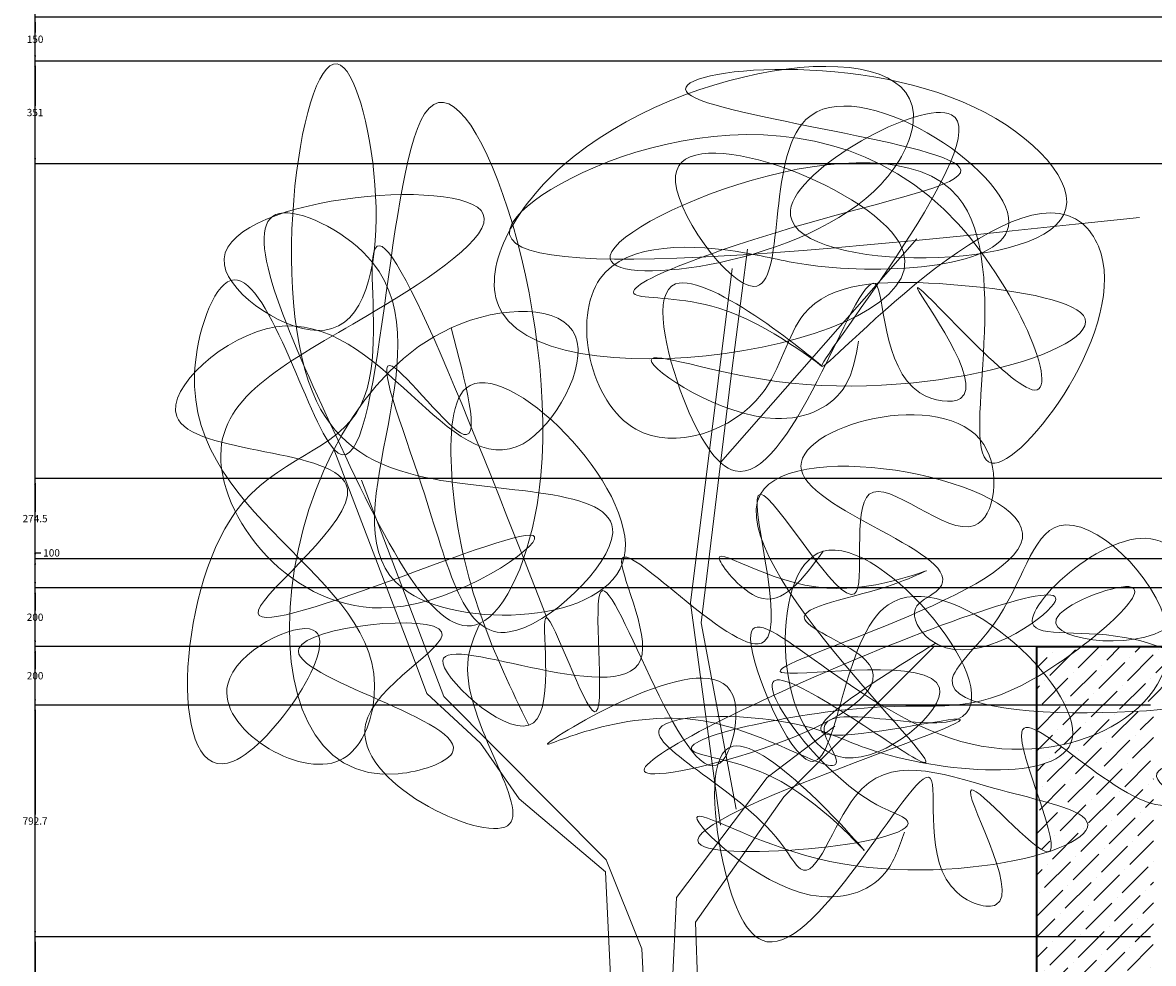
# Model space of a CAD drawing. Units: millimetres. Extents: x -692 to 9639, y -141 to 10345.
# Tile 2 of 19: x -692 to 3174, y 1765 to 4981. Entities that reach past the tile are written whole.
import ezdxf

# ---------------------------------------------------------------- set-up
doc = ezdxf.new("R2010")
doc.units = ezdxf.units.MM
doc.header["$MEASUREMENT"] = 0
for name, color, linetype, lineweight in [('A-ANNO-DIMS', 2, 'Continuous', 18), ('A-ELEV', 7, 'Continuous', 35), ('A-ELEV-PATT', 8, 'Continuous', 13), ('L-PLNT', 3, 'Continuous', 18)]:
    doc.layers.add(name, color=color, linetype=linetype, lineweight=lineweight)
doc.styles.get("Standard").update_dxf_attribs({"font": 'arial.ttf'})
doc.dimstyles.get("Standard").update_dxf_attribs({"dimtxt": 25, "dimasz": 20, "dimexe": 0.18, "dimexo": 10, "dimgap": 10, "dimtad": 0, "dimtih": 1, "dimtoh": 1, "dimdec": 0, "dimzin": 0, "dimdsep": 46, "dimtxsty": 'Standard', "dimcen": 10, "dimadec": 0, "dimazin": 0, "dimtfac": 1, "dimtdec": 0, "dimtofl": 0, "dimtmove": 0, "dimatfit": 3, "dimfxl": 1, "dimtolj": 1, "dimtzin": 0, "dimarcsym": 0})

# ---------------------------------------------------------------- blocks, each defined once
blk = doc.blocks.new('*D7')
at = {"layer": 'A-ANNO-DIMS', "color": 0, "lineweight": -2, "transparency": 16777216}
for p, q in [((8481.5, 9848.8), (-649.1, 9848.8)), ((-648.9, 9828.8), (-648.9, 5124.9)), ((-648.9, 375.6), (-648.9, 5079.4)), ((2463.7, 355.6), (-649.1, 355.6))]:
    blk.add_line(p, q, dxfattribs=at)
at = {"layer": 'A-ANNO-DIMS', "color": 0, "lineweight": -3, "transparency": 16777216}
for points in [[(-652.2, 9828.8), (-645.6, 9828.8), (-648.9, 9848.8)], [(-652.2, 375.6), (-645.6, 375.6), (-648.9, 355.6)]]:
    blk.add_solid(points, dxfattribs=at)
at = {"layer": 'Defpoints', "color": 0, "lineweight": -3, "transparency": 16777216}
for p in [(-648.9, 9848.8), (8491.5, 9848.8), (2473.7, 355.6)]:
    blk.add_point(p, dxfattribs=at)
at = {"layer": 'A-ANNO-DIMS', "color": 0, "transparency": 16777216, "insert": (-648.9, 5102.2), "char_height": 25, "attachment_point": 5}
blk.add_mtext('\\A1;9493', dxfattribs=at)
blk = doc.blocks.new('*D25')
at = {"layer": 'A-ANNO-DIMS', "color": 0, "lineweight": -2, "transparency": 16777216}
for p, q in [((3163.7, 1855.6), (-649.1, 1855.6)), ((-648.9, 1835.6), (-648.9, 1378.3)), ((-648.9, 875.6), (-648.9, 1332.8)), ((2763.7, 855.6), (-649.1, 855.6))]:
    blk.add_line(p, q, dxfattribs=at)
at = {"layer": 'A-ANNO-DIMS', "color": 0, "lineweight": -3, "transparency": 16777216}
for points in [[(-652.2, 1835.6), (-645.6, 1835.6), (-648.9, 1855.6)], [(-652.2, 875.6), (-645.6, 875.6), (-648.9, 855.6)]]:
    blk.add_solid(points, dxfattribs=at)
at = {"layer": 'Defpoints', "color": 0, "lineweight": -3, "transparency": 16777216}
for p in [(-648.9, 1855.6), (3173.7, 1855.6), (2773.7, 855.6)]:
    blk.add_point(p, dxfattribs=at)
at = {"layer": 'A-ANNO-DIMS', "color": 0, "transparency": 16777216, "insert": (-648.9, 1355.6), "char_height": 25, "attachment_point": 5}
blk.add_mtext('\\A1;1000', dxfattribs=at)
blk = doc.blocks.new('*D26')
at = {"layer": 'A-ANNO-DIMS', "color": 0, "lineweight": -2, "transparency": 16777216}
for p, q in [((3163.7, 2648.3), (-649.1, 2648.3)), ((-648.9, 2628.3), (-648.9, 2274.7)), ((-648.9, 1875.6), (-648.9, 2229.2)), ((3163.7, 1855.6), (-649.1, 1855.6))]:
    blk.add_line(p, q, dxfattribs=at)
at = {"layer": 'A-ANNO-DIMS', "color": 0, "lineweight": -3, "transparency": 16777216}
for points in [[(-652.2, 2628.3), (-645.6, 2628.3), (-648.9, 2648.3)], [(-652.2, 1875.6), (-645.6, 1875.6), (-648.9, 1855.6)]]:
    blk.add_solid(points, dxfattribs=at)
at = {"layer": 'Defpoints', "color": 0, "lineweight": -3, "transparency": 16777216}
for p in [(-648.9, 2648.3), (3173.7, 2648.3), (3173.7, 1855.6)]:
    blk.add_point(p, dxfattribs=at)
at = {"layer": 'A-ANNO-DIMS', "color": 0, "transparency": 16777216, "insert": (-648.9, 2251.9), "char_height": 25, "attachment_point": 5}
blk.add_mtext('\\A1;792.7', dxfattribs=at)
blk = doc.blocks.new('*D27')
at = {"layer": 'A-ANNO-DIMS', "color": 0, "lineweight": -2, "transparency": 16777216}
for p, q in [((2763.7, 2848.3), (-649.1, 2848.3)), ((-648.9, 2828.3), (-648.9, 2771)), ((-648.9, 2668.3), (-648.9, 2725.5)), ((3163.7, 2648.3), (-649.1, 2648.3))]:
    blk.add_line(p, q, dxfattribs=at)
at = {"layer": 'A-ANNO-DIMS', "color": 0, "lineweight": -3, "transparency": 16777216}
for points in [[(-652.2, 2828.3), (-645.6, 2828.3), (-648.9, 2848.3)], [(-652.2, 2668.3), (-645.6, 2668.3), (-648.9, 2648.3)]]:
    blk.add_solid(points, dxfattribs=at)
at = {"layer": 'Defpoints', "color": 0, "lineweight": -3, "transparency": 16777216}
for p in [(-648.9, 2848.3), (2773.7, 2848.3), (3173.7, 2648.3)]:
    blk.add_point(p, dxfattribs=at)
at = {"layer": 'A-ANNO-DIMS', "color": 0, "transparency": 16777216, "insert": (-648.9, 2748.3), "char_height": 25, "attachment_point": 5}
blk.add_mtext('\\A1;200', dxfattribs=at)
blk = doc.blocks.new('*D59')
at = {"layer": 'A-ANNO-DIMS', "color": 0, "lineweight": -2, "transparency": 16777216}
for p, q in [((5031.5, 3048.3), (-649.1, 3048.3)), ((-648.9, 3028.3), (-648.9, 2971)), ((-648.9, 2868.3), (-648.9, 2925.5)), ((3181.5, 2848.3), (-649.1, 2848.3))]:
    blk.add_line(p, q, dxfattribs=at)
at = {"layer": 'A-ANNO-DIMS', "color": 0, "lineweight": -3, "transparency": 16777216}
for points in [[(-652.2, 3028.3), (-645.6, 3028.3), (-648.9, 3048.3)], [(-652.2, 2868.3), (-645.6, 2868.3), (-648.9, 2848.3)]]:
    blk.add_solid(points, dxfattribs=at)
at = {"layer": 'Defpoints', "color": 0, "lineweight": -3, "transparency": 16777216}
for p in [(-648.9, 3048.3), (5041.5, 3048.3), (3191.5, 2848.3)]:
    blk.add_point(p, dxfattribs=at)
at = {"layer": 'A-ANNO-DIMS', "color": 0, "transparency": 16777216, "insert": (-648.9, 2948.3), "char_height": 25, "attachment_point": 5}
blk.add_mtext('\\A1;200', dxfattribs=at)
blk = doc.blocks.new('*D60')
at = {"layer": 'A-ANNO-DIMS', "color": 0, "lineweight": -2, "transparency": 16777216}
for p, q in [((5031.5, 3148.3), (-649.1, 3148.3)), ((-648.9, 3148.3), (-648.9, 3168.3)), ((-648.9, 3168.3), (-628.9, 3168.3)), ((-648.9, 3068.3), (-648.9, 3128.3)), ((5031.5, 3048.3), (-649.1, 3048.3))]:
    blk.add_line(p, q, dxfattribs=at)
at = {"layer": 'A-ANNO-DIMS', "color": 0, "lineweight": -3, "transparency": 16777216}
for points in [[(-652.2, 3128.3), (-645.6, 3128.3), (-648.9, 3148.3)], [(-652.2, 3068.3), (-645.6, 3068.3), (-648.9, 3048.3)]]:
    blk.add_solid(points, dxfattribs=at)
at = {"layer": 'Defpoints', "color": 0, "lineweight": -3, "transparency": 16777216}
for p in [(-648.9, 3148.3), (5041.5, 3148.3), (5041.5, 3048.3)]:
    blk.add_point(p, dxfattribs=at)
at = {"layer": 'A-ANNO-DIMS', "color": 0, "transparency": 16777216, "insert": (-592.5, 3168.3), "char_height": 25, "attachment_point": 5}
blk.add_mtext('\\A1;100', dxfattribs=at)
blk = doc.blocks.new('*D61')
at = {"layer": 'A-ANNO-DIMS', "color": 0, "lineweight": -2, "transparency": 16777216}
for p, q in [((3931.5, 3422.8), (-649.1, 3422.8)), ((-648.9, 3402.8), (-648.9, 3308.3)), ((-648.9, 3168.3), (-648.9, 3262.8)), ((5031.5, 3148.3), (-649.1, 3148.3))]:
    blk.add_line(p, q, dxfattribs=at)
at = {"layer": 'A-ANNO-DIMS', "color": 0, "lineweight": -3, "transparency": 16777216}
for points in [[(-652.2, 3402.8), (-645.6, 3402.8), (-648.9, 3422.8)], [(-652.2, 3168.3), (-645.6, 3168.3), (-648.9, 3148.3)]]:
    blk.add_solid(points, dxfattribs=at)
at = {"layer": 'Defpoints', "color": 0, "lineweight": -3, "transparency": 16777216}
for p in [(-648.9, 3422.8), (3941.5, 3422.8), (5041.5, 3148.3)]:
    blk.add_point(p, dxfattribs=at)
at = {"layer": 'A-ANNO-DIMS', "color": 0, "transparency": 16777216, "insert": (-648.9, 3285.5), "char_height": 25, "attachment_point": 5}
blk.add_mtext('\\A1;274.5', dxfattribs=at)
blk = doc.blocks.new('*D62')
at = {"layer": 'A-ANNO-DIMS', "color": 0, "lineweight": -2, "transparency": 16777216}
for p, q in [((3781.5, 4848.8), (-649.1, 4848.8)), ((-648.9, 4828.8), (-648.9, 4696)), ((-648.9, 4517.8), (-648.9, 4650.5)), ((3931.5, 4497.8), (-649.1, 4497.8))]:
    blk.add_line(p, q, dxfattribs=at)
at = {"layer": 'A-ANNO-DIMS', "color": 0, "lineweight": -3, "transparency": 16777216}
for points in [[(-652.2, 4828.8), (-645.6, 4828.8), (-648.9, 4848.8)], [(-652.2, 4517.8), (-645.6, 4517.8), (-648.9, 4497.8)]]:
    blk.add_solid(points, dxfattribs=at)
at = {"layer": 'Defpoints', "color": 0, "lineweight": -3, "transparency": 16777216}
for p in [(-648.9, 4848.8), (3791.5, 4848.8), (3941.5, 4497.8)]:
    blk.add_point(p, dxfattribs=at)
at = {"layer": 'A-ANNO-DIMS', "color": 0, "transparency": 16777216, "insert": (-648.9, 4673.3), "char_height": 25, "attachment_point": 5}
blk.add_mtext('\\A1;351', dxfattribs=at)
blk = doc.blocks.new('*D63')
at = {"layer": 'A-ANNO-DIMS', "color": 0, "lineweight": -2, "transparency": 16777216}
for p, q in [((3931.5, 4998.8), (-649.1, 4998.8)), ((-648.9, 4978.8), (-648.9, 4946.5)), ((-648.9, 4868.8), (-648.9, 4901)), ((3781.5, 4848.8), (-649.1, 4848.8))]:
    blk.add_line(p, q, dxfattribs=at)
at = {"layer": 'A-ANNO-DIMS', "color": 0, "lineweight": -3, "transparency": 16777216}
for points in [[(-652.2, 4978.8), (-645.6, 4978.8), (-648.9, 4998.8)], [(-652.2, 4868.8), (-645.6, 4868.8), (-648.9, 4848.8)]]:
    blk.add_solid(points, dxfattribs=at)
at = {"layer": 'Defpoints', "color": 0, "lineweight": -3, "transparency": 16777216}
for p in [(-648.9, 4998.8), (3941.5, 4998.8), (3791.5, 4848.8)]:
    blk.add_point(p, dxfattribs=at)
at = {"layer": 'A-ANNO-DIMS', "color": 0, "transparency": 16777216, "insert": (-648.9, 4923.8), "char_height": 25, "attachment_point": 5}
blk.add_mtext('\\A1;150', dxfattribs=at)

msp = doc.modelspace()

# ---------------------------------------------------------------- hatches: boundary and pattern name
at = {"layer": 'A-ELEV-PATT'}
h = msp.add_hatch(dxfattribs=at)
h.set_pattern_fill('ANSI36', color=256, scale=400)
edge = h.paths.add_edge_path()
edge.add_spline(control_points=[(3173.746, 2309.965), (3085.901, 2332.226), (2969.139, 2424.713), (2876.436, 2493.45)], knot_values=[20955.88576955, 20955.88576955, 20955.88576955, 20955.88576955, 21219.85539585, 21219.85539585, 21219.85539585, 21219.85539585], degree=3, periodic=0)
edge.add_spline(control_points=[(2876.436, 2493.45), (2855.134, 2468.311), (2819.135, 2451.154), (2773.746, 2440.514)], knot_values=[5238.08213467, 5238.08213467, 5238.08213467, 5238.08213467, 5382.8513026, 5382.8513026, 5382.8513026, 5382.8513026], degree=3, periodic=0)
edge.add_line((2773.746, 2440.514), (2773.746, 2354.397))
edge.add_spline(control_points=[(2773.746, 2354.397), (2777.278, 2343.918), (2780.812, 2333.449), (2784.279, 2323.093)], knot_values=[20514.20511429, 20514.20511429, 20514.20511429, 20514.20511429, 20537.39604293, 20537.39604293, 20537.39604293, 20537.39604293], degree=3, periodic=0)
edge.add_spline(control_points=[(2784.279, 2323.093), (2849.257, 2305.468), (3007.384, 2255.171), (2928.441, 2185.016), (2819.76, 2148.371)], knot_values=[1896.27813718, 1896.27813718, 1896.27813718, 1896.27813718, 2077.70067144, 2424.51760392, 2424.51760392, 2424.51760392, 2424.51760392], degree=3, periodic=0)
edge.add_spline(control_points=[(2819.76, 2148.371), (2817.899, 2146.748), (2815.52, 2145.926), (2812.57, 2145.987)], knot_values=[20304.87329269, 20304.87329269, 20304.87329269, 20304.87329269, 20326.21847821, 20326.21847821, 20326.21847821, 20326.21847821], degree=3, periodic=0)
edge.add_spline(control_points=[(2812.57, 2145.987), (2800.291, 2141.985), (2787.329, 2138.102), (2773.746, 2134.363)], knot_values=[1850.39591646, 1850.39591646, 1850.39591646, 1850.39591646, 1888.716341, 1888.716341, 1888.716341, 1888.716341], degree=3, periodic=0)
edge.add_line((2773.746, 2134.363), (2773.746, 855.575))
edge.add_line((2773.746, 855.575), (3173.746, 855.575))
edge.add_line((3173.746, 855.575), (3173.746, 2309.965))
edge = h.paths.add_edge_path()
edge.add_spline(control_points=[(3420.651, 2717.101), (3368.378, 2761.363), (3299.425, 2803.396), (3225.3, 2834.508)], knot_values=[12552.99587302, 12552.99587302, 12552.99587302, 12552.99587302, 12712.02358035, 12712.02358035, 12712.02358035, 12712.02358035], degree=3, periodic=0)
edge.add_spline(control_points=[(3225.3, 2834.508), (3218.267, 2754.576), (3174.644, 2682.922), (3107.112, 2626.403)], knot_values=[8572.46293399, 8572.46293399, 8572.46293399, 8572.46293399, 8814.86919927, 8814.86919927, 8814.86919927, 8814.86919927], degree=3, periodic=0)
edge.add_spline(control_points=[(3107.112, 2626.403), (3129.755, 2627.593), (3152.034, 2628.996), (3173.746, 2630.586)], knot_values=[10558.19039557, 10558.19039557, 10558.19039557, 10558.19039557, 10599.03834951, 10599.03834951, 10599.03834951, 10599.03834951], degree=3, periodic=0)
edge.add_line((3173.746, 2630.586), (3173.746, 2648.27))
edge.add_line((3173.746, 2648.27), (3219.774, 2648.27))
edge.add_spline(control_points=[(3219.774, 2648.27), (3215.509, 2669.279), (3223.352, 2735.229), (3357.845, 2728.872), (3420.651, 2717.101)], knot_values=[11042.13010686, 11042.13010686, 11042.13010686, 11042.13010686, 11110.4948836, 11298.41454305, 11298.41454305, 11298.41454305, 11298.41454305], degree=3, periodic=0)
edge = h.paths.add_edge_path()
edge.add_spline(control_points=[(3107.112, 2626.403), (3174.644, 2682.922), (3218.267, 2754.576), (3225.3, 2834.508)], knot_values=[8572.46293399, 8572.46293399, 8572.46293399, 8572.46293399, 8814.86919927, 8814.86919927, 8814.86919927, 8814.86919927], degree=3, periodic=0)
edge.add_spline(control_points=[(3225.3, 2834.508), (3213.709, 2839.374), (3201.991, 2843.972), (3190.19, 2848.27)], knot_values=[12712.02358035, 12712.02358035, 12712.02358035, 12712.02358035, 12736.8923557, 12736.8923557, 12736.8923557, 12736.8923557], degree=3, periodic=0)
edge.add_line((3190.19, 2848.27), (2928.387, 2848.27))
edge.add_spline(control_points=[(2928.387, 2848.27), (2886.081, 2816.098), (2840.884, 2784.767), (2798.089, 2758.256)], knot_values=[14939.29716066, 14939.29716066, 14939.29716066, 14939.29716066, 15046.25935392, 15046.25935392, 15046.25935392, 15046.25935392], degree=3, periodic=0)
edge.add_spline(control_points=[(2798.089, 2758.256), (2836.427, 2711.897), (2866.292, 2664.879), (2883.022, 2622.327)], knot_values=[5561.23366662, 5561.23366662, 5561.23366662, 5561.23366662, 5704.57044689, 5704.57044689, 5704.57044689, 5704.57044689], degree=3, periodic=0)
edge.add_spline(control_points=[(2883.022, 2622.327), (2956.927, 2620.92), (3033.919, 2622.554), (3107.112, 2626.403)], knot_values=[10426.14846168, 10426.14846168, 10426.14846168, 10426.14846168, 10558.19039557, 10558.19039557, 10558.19039557, 10558.19039557], degree=3, periodic=0)
edge = h.paths.add_edge_path()
edge.add_spline(control_points=[(3173.746, 2630.586), (3152.034, 2628.996), (3129.755, 2627.593), (3107.112, 2626.403)], knot_values=[10558.19039557, 10558.19039557, 10558.19039557, 10558.19039557, 10599.03834951, 10599.03834951, 10599.03834951, 10599.03834951], degree=3, periodic=0)
edge.add_spline(control_points=[(3107.112, 2626.403), (3049.969, 2578.578), (2975.708, 2541.59), (2892.012, 2519.592)], knot_values=[8367.34849038, 8367.34849038, 8367.34849038, 8367.34849038, 8572.46293399, 8572.46293399, 8572.46293399, 8572.46293399], degree=3, periodic=0)
edge.add_spline(control_points=[(2892.012, 2519.592), (2888.384, 2510.058), (2883.137, 2501.359), (2876.436, 2493.45)], knot_values=[5382.8513026, 5382.8513026, 5382.8513026, 5382.8513026, 5428.39625745, 5428.39625745, 5428.39625745, 5428.39625745], degree=3, periodic=0)
edge.add_spline(control_points=[(2876.436, 2493.45), (2969.139, 2424.713), (3085.901, 2332.226), (3173.746, 2309.965)], knot_values=[20955.88576955, 20955.88576955, 20955.88576955, 20955.88576955, 21219.85539585, 21219.85539585, 21219.85539585, 21219.85539585], degree=3, periodic=0)
edge.add_line((3173.746, 2309.965), (3173.746, 2630.586))
edge = h.paths.add_edge_path(flags=17)
edge.add_spline(control_points=[(2819.76, 2148.371), (2928.441, 2185.016), (3007.384, 2255.171), (2849.257, 2305.468), (2784.279, 2323.093)], knot_values=[1896.27813718, 1896.27813718, 1896.27813718, 1896.27813718, 2243.09506965, 2424.51760392, 2424.51760392, 2424.51760392, 2424.51760392], degree=3, periodic=0)
edge.add_spline(control_points=[(2784.279, 2323.093), (2812.387, 2239.151), (2836.152, 2162.664), (2819.76, 2148.371)], knot_values=[20326.21847821, 20326.21847821, 20326.21847821, 20326.21847821, 20514.20511429, 20514.20511429, 20514.20511429, 20514.20511429], degree=3, periodic=0)
edge = h.paths.add_edge_path(flags=17)
edge.add_spline(control_points=[(2819.76, 2148.371), (2836.152, 2162.664), (2812.387, 2239.151), (2784.279, 2323.093)], knot_values=[20326.21847821, 20326.21847821, 20326.21847821, 20326.21847821, 20514.20511429, 20514.20511429, 20514.20511429, 20514.20511429], degree=3, periodic=0)
edge.add_spline(control_points=[(2784.279, 2323.093), (2780.798, 2324.038), (2777.286, 2324.983), (2773.746, 2325.93)], knot_values=[2424.51760392, 2424.51760392, 2424.51760392, 2424.51760392, 2434.23800618, 2434.23800618, 2434.23800618, 2434.23800618], degree=3, periodic=0)
edge.add_line((2773.746, 2325.93), (2773.746, 2166.486))
edge.add_spline(control_points=[(2773.746, 2166.486), (2790.303, 2153.967), (2803.9, 2146.166), (2812.57, 2145.987)], knot_values=[20242.12265912, 20242.12265912, 20242.12265912, 20242.12265912, 20304.87329269, 20304.87329269, 20304.87329269, 20304.87329269], degree=3, periodic=0)
edge.add_spline(control_points=[(2812.57, 2145.987), (2814.994, 2146.777), (2817.39, 2147.572), (2819.76, 2148.371)], knot_values=[1888.716341, 1888.716341, 1888.716341, 1888.716341, 1896.27813718, 1896.27813718, 1896.27813718, 1896.27813718], degree=3, periodic=0)
edge = h.paths.add_edge_path()
edge.add_spline(control_points=[(2892.012, 2519.592), (2893.653, 2523.907), (2902.094, 2552.818), (2896.12, 2589.012), (2883.022, 2622.327)], knot_values=[5428.39625745, 5428.39625745, 5428.39625745, 5428.39625745, 5449.01011401, 5561.23366662, 5561.23366662, 5561.23366662, 5561.23366662], degree=3, periodic=0)
edge.add_spline(control_points=[(2883.022, 2622.327), (2845.501, 2623.042), (2808.775, 2624.54), (2773.746, 2626.93)], knot_values=[10359.11175247, 10359.11175247, 10359.11175247, 10359.11175247, 10426.14846168, 10426.14846168, 10426.14846168, 10426.14846168], degree=3, periodic=0)
edge.add_line((2773.746, 2626.93), (2773.746, 2561.8))
edge.add_spline(control_points=[(2773.746, 2561.8), (2795.257, 2551.206), (2822.448, 2532.82), (2853.096, 2510.59)], knot_values=[20841.44589883, 20841.44589883, 20841.44589883, 20841.44589883, 20933.19502211, 20933.19502211, 20933.19502211, 20933.19502211], degree=3, periodic=0)
edge.add_spline(control_points=[(2853.096, 2510.59), (2866.269, 2513.232), (2879.25, 2516.238), (2892.012, 2519.592)], knot_values=[8336.07392909, 8336.07392909, 8336.07392909, 8336.07392909, 8367.34849038, 8367.34849038, 8367.34849038, 8367.34849038], degree=3, periodic=0)
edge = h.paths.add_edge_path(flags=17)
edge.add_spline(control_points=[(2892.012, 2519.592), (2975.708, 2541.59), (3049.969, 2578.578), (3107.112, 2626.403)], knot_values=[8367.34849038, 8367.34849038, 8367.34849038, 8367.34849038, 8572.46293399, 8572.46293399, 8572.46293399, 8572.46293399], degree=3, periodic=0)
edge.add_spline(control_points=[(3107.112, 2626.403), (3033.919, 2622.554), (2956.927, 2620.92), (2883.022, 2622.327)], knot_values=[10426.14846168, 10426.14846168, 10426.14846168, 10426.14846168, 10558.19039557, 10558.19039557, 10558.19039557, 10558.19039557], degree=3, periodic=0)
edge.add_spline(control_points=[(2883.022, 2622.327), (2896.12, 2589.012), (2902.094, 2552.818), (2893.653, 2523.907), (2892.012, 2519.592)], knot_values=[5428.39625745, 5428.39625745, 5428.39625745, 5428.39625745, 5540.61981006, 5561.23366662, 5561.23366662, 5561.23366662, 5561.23366662], degree=3, periodic=0)
edge = h.paths.add_edge_path()
edge.add_spline(control_points=[(2773.746, 2440.514), (2819.135, 2451.154), (2855.134, 2468.311), (2876.436, 2493.45)], knot_values=[5238.08213467, 5238.08213467, 5238.08213467, 5238.08213467, 5382.8513026, 5382.8513026, 5382.8513026, 5382.8513026], degree=3, periodic=0)
edge.add_spline(control_points=[(2876.436, 2493.45), (2868.467, 2499.359), (2860.676, 2505.092), (2853.096, 2510.59)], knot_values=[20933.19502211, 20933.19502211, 20933.19502211, 20933.19502211, 20955.88576955, 20955.88576955, 20955.88576955, 20955.88576955], degree=3, periodic=0)
edge.add_spline(control_points=[(2853.096, 2510.59), (2827.314, 2505.418), (2800.796, 2501.637), (2773.746, 2499.359)], knot_values=[8274.86392127, 8274.86392127, 8274.86392127, 8274.86392127, 8336.07392909, 8336.07392909, 8336.07392909, 8336.07392909], degree=3, periodic=0)
edge.add_line((2773.746, 2499.359), (2773.746, 2440.514))
edge = h.paths.add_edge_path()
edge.add_spline(control_points=[(2883.022, 2622.327), (2866.292, 2664.879), (2836.427, 2711.897), (2798.089, 2758.256)], knot_values=[5561.23366662, 5561.23366662, 5561.23366662, 5561.23366662, 5704.57044689, 5704.57044689, 5704.57044689, 5704.57044689], degree=3, periodic=0)
edge.add_spline(control_points=[(2798.089, 2758.256), (2789.874, 2753.166), (2781.747, 2748.254), (2773.746, 2743.548)], knot_values=[15046.25935392, 15046.25935392, 15046.25935392, 15046.25935392, 15066.79294618, 15066.79294618, 15066.79294618, 15066.79294618], degree=3, periodic=0)
edge.add_line((2773.746, 2743.548), (2773.746, 2626.93))
edge.add_spline(control_points=[(2773.746, 2626.93), (2808.775, 2624.54), (2845.501, 2623.042), (2883.022, 2622.327)], knot_values=[10359.11175247, 10359.11175247, 10359.11175247, 10359.11175247, 10426.14846168, 10426.14846168, 10426.14846168, 10426.14846168], degree=3, periodic=0)
edge = h.paths.add_edge_path()
edge.add_spline(control_points=[(2798.089, 2758.256), (2840.884, 2784.767), (2886.081, 2816.098), (2928.387, 2848.27)], knot_values=[14939.29716066, 14939.29716066, 14939.29716066, 14939.29716066, 15046.25935392, 15046.25935392, 15046.25935392, 15046.25935392], degree=3, periodic=0)
edge.add_line((2928.387, 2848.27), (2773.746, 2848.27))
edge.add_line((2773.746, 2848.27), (2773.746, 2786.349))
edge.add_spline(control_points=[(2773.746, 2786.349), (2782.183, 2777.04), (2790.311, 2767.662), (2798.089, 2758.256)], knot_values=[5704.57044689, 5704.57044689, 5704.57044689, 5704.57044689, 5733.65273084, 5733.65273084, 5733.65273084, 5733.65273084], degree=3, periodic=0)
edge = h.paths.add_edge_path()
edge.add_spline(control_points=[(3463.702, 2676.006), (3451.141, 2689.747), (3436.681, 2703.529), (3420.651, 2717.101)], knot_values=[12504.23047843, 12504.23047843, 12504.23047843, 12504.23047843, 12552.99587302, 12552.99587302, 12552.99587302, 12552.99587302], degree=3, periodic=0)
edge.add_spline(control_points=[(3420.651, 2717.101), (3357.845, 2728.872), (3223.352, 2735.229), (3215.509, 2669.279), (3219.774, 2648.27)], knot_values=[11042.13010686, 11042.13010686, 11042.13010686, 11042.13010686, 11230.04976631, 11298.41454305, 11298.41454305, 11298.41454305, 11298.41454305], degree=3, periodic=0)
edge.add_line((3219.774, 2648.27), (3341.426, 2648.27))
edge.add_spline(control_points=[(3341.426, 2648.27), (3397.595, 2656.506), (3440.895, 2666.057), (3463.702, 2676.006)], knot_values=[10715.9300286, 10715.9300286, 10715.9300286, 10715.9300286, 10852.53626518, 10852.53626518, 10852.53626518, 10852.53626518], degree=3, periodic=0)
edge = h.paths.add_edge_path()
edge.add_spline(control_points=[(2853.096, 2510.59), (2822.448, 2532.82), (2795.257, 2551.206), (2773.746, 2561.8)], knot_values=[20841.44589883, 20841.44589883, 20841.44589883, 20841.44589883, 20933.19502211, 20933.19502211, 20933.19502211, 20933.19502211], degree=3, periodic=0)
edge.add_line((2773.746, 2561.8), (2773.746, 2499.359))
edge.add_spline(control_points=[(2773.746, 2499.359), (2800.796, 2501.637), (2827.314, 2505.418), (2853.096, 2510.59)], knot_values=[8274.86392127, 8274.86392127, 8274.86392127, 8274.86392127, 8336.07392909, 8336.07392909, 8336.07392909, 8336.07392909], degree=3, periodic=0)

# ---------------------------------------------------------------- linework, layer by layer
at = {"layer": 'A-ELEV'}
for q in [(2773.746, 855.575), (5773.746, 2848.27)]:
    msp.add_line((2773.746, 2848.27), q, dxfattribs=at)
at = {"layer": 'L-PLNT'}
for p, q in [((1694.41, 3476.755), (2365.48, 4241.188)), ((1728.336, 3755.462), (1786.517, 4206.053)), ((1734.079, 4140.36), (1591.815, 2997.988)), ((1627.703, 2928.757), (1728.336, 3755.462)), ((646.36, 2803.345), (372.582, 3522.228)), ((466.943, 3417.172), (748.756, 2677.189)), ((1591.815, 2997.988), (1694.591, 2237.165)), ((1747.838, 2291.806), (1627.703, 2928.757)), ((1910.853, 2334.669), (2422.639, 2846.042)), ((690.463, 2687.541), (646.36, 2803.345)), ((873.763, 2517.546), (690.463, 2687.541)), ((748.756, 2677.189), (1303.638, 2119.721)), ((1853.307, 2400.038), (2084.447, 2576.177)), ((1005.385, 2327.197), (873.763, 2517.546)), ((1543.202, 1990.116), (1853.307, 2400.038)), ((1301.056, 2077.694), (1005.385, 2327.197)), ((1608.333, 1905.92), (1910.853, 2334.669)), ((1303.638, 2119.721), (1424.921, 1814.529)), ((1301.056, 2077.694), (1317.991, 1721.29)), ((1512.588, 1320.381), (1543.202, 1990.116)), ((1668.259, 355.575), (1608.333, 1905.92)), ((1468.429, 1029.289), (1424.921, 1814.529))]:
    msp.add_line(p, q, dxfattribs=at)
for points, knots in [([(773.155, 3937.484), (823.676, 3746.696), (920.778, 3380.004), (438.152, 4023.063), (733.257, 3283.516), (852.426, 2673.934), (1621.551, 3415.579), (658.912, 3350.046), (83.123, 3754.796), (387.973, 5649.892), (660.326, 3619.622), (-430.212, 4344.4), (1298.576, 4507.959), (405.521, 3907.951), (-261.937, 3601.368), (404.911, 2721.405), (1564.953, 3531.288), (-432.999, 2606.763), (807.942, 3554.364), (-480.906, 3478.784), (412.834, 4286.391), (873.838, 3140.074), (1356.141, 4017.079), (192.159, 4014.414), (-15.546, 2191.416), (1038.42, 2544.512), (-272.623, 2860.496), (1070.695, 2999.253), (138.34, 2529.078), (1295.949, 1978.694), (756.735, 2666.695), (852.776, 2883.872), (872.242, 2927.891)], [0, 0, 0, 0, 366.84674553, 705.0755833, 1127.60687806, 1708.56019235, 2198.09683598, 2891.77747969, 3350.55771939, 4464.55955871, 5362.87921941, 5772.09298323, 6674.14140748, 7170.704565, 7878.38687444, 8671.28078344, 9219.77836303, 10196.69914934, 10711.16636685, 11344.7041634, 11801.14382375, 12735.71627216, 13144.72100701, 13571.01650674, 15105.84793506, 15302.71088156, 15937.2400277, 16428.59100295, 16838.26205876, 17433.91047945, 18003.85099419, 18148.7356522, 18148.7356522, 18148.7356522, 18148.7356522]), ([(2165.754, 3891.475), (2156.454, 3838.257), (2131.336, 3694.529), (1828.981, 3544.556), (1234.462, 3939.765), (2171.187, 3600.974), (3342.978, 3968.878), (2432.599, 4108.039), (1950.724, 4089.121), (1875.104, 3632.281), (1299.63, 3434.838), (1128.38, 4245.511), (1713.167, 4218.345), (2113.861, 4110.074), (3149.615, 4165.738), (1761.636, 5086.777), (1972.132, 3739.817), (1194.577, 4794.7), (3283.569, 4019.583), (613.423, 3576.192), (1194.213, 4802.087), (2547.188, 4984.273), (2147.699, 4173.884), (527.708, 3974.57), (2970.374, 5004.952), (2318.591, 2908.941), (3140.144, 4006.979), (2748.192, 4569.184), (1417.574, 3067.47), (3032.493, 5075.529), (1319.076, 4138.415), (3212.15, 4112.243), (2458.355, 4927.6), (847.163, 4747.765), (2972.807, 4514.335), (1976.467, 4316.336), (1175.361, 4020.027), (1737.289, 4053.993), (2300.005, 3591.209), (1396.914, 4348.25), (1537.361, 3704.647), (1763.319, 3319.271), (2024.288, 3715.779), (2272.185, 4311.535), (2237.928, 3709.962), (2670.254, 3653.157), (2113.766, 4390.234), (3002.683, 3357.462), (2332.138, 5008.934), (-42.634, 3979.162), (1956.694, 4190.614), (3126.741, 4314.36)], [0, 0, 0, 0, 156.01346293, 421.35741543, 891.47725045, 1326.49022079, 2392.20438866, 2885.8478872, 3358.96684665, 3669.49719622, 4115.61990814, 4644.55411056, 5145.83540445, 5376.12253264, 6069.20829618, 6847.01771902, 7444.00308071, 7908.15080043, 8706.97525164, 10085.92062572, 10629.27654129, 11837.49964897, 12076.37300863, 13037.3913742, 14244.31810109, 15161.81230822, 15987.7709146, 16082.64489186, 17097.97008769, 18064.75232597, 18704.4498569, 19639.49855139, 20117.66518754, 21095.82849536, 22062.69089297, 22623.83614076, 23250.51210285, 23533.88270994, 23937.98896772, 24510.82194297, 24906.15111226, 25207.57810477, 25623.06805775, 26010.11826538, 26412.08156501, 26552.338364, 26953.95880093, 27464.88681372, 28078.27224563, 29587.51362547, 31716.9300752, 31716.9300752, 31716.9300752, 31716.9300752]), ([(1100.092, 2946.557), (807.023, 3696.593), (409.192, 4714.745), (569.925, 3530.51), (-152.775, 3465.055), (-208.104, 1952.866), (548.549, 3087.84), (-235.684, 2696.746), (380.488, 2316.733), (705.193, 3047.745), (-314.229, 3311.036), (72.51, 4397.522), (525.726, 2714.442), (560.229, 5720.429), (1270.529, 3655.977), (818.077, 2651.18), (390.599, 3525.426), (-37.865, 4493.924), (898.609, 4020.94), (36.217, 2865.508), (1854.536, 2949.623), (773.839, 4035.261), (761.475, 3153.016), (921.686, 2820.945), (1038.352, 2579.131)], [0, 0, 0, 0, 1345.84516735, 1826.94294504, 2390.16850477, 3242.22549087, 3767.30674542, 4113.6768489, 4576.99642791, 4787.97180678, 6086.44701257, 6424.37697059, 7100.7508866, 8288.65931334, 9641.46014173, 10130.45306753, 10981.67154523, 11721.43710257, 12070.10722531, 13188.44774419, 13953.15192659, 14744.19070929, 15069.29570079, 15940.30052044, 15940.30052044, 15940.30052044, 15940.30052044]), ([(2044.996, 3173.747), (1976.435, 3079.963), (1861.652, 2922.954), (1574.026, 3271.049), (2022.896, 2935.029), (2502.669, 3155.818), (2212.968, 3021.247), (1817.534, 2968.505), (2599.158, 2691.745), (202.738, 2002.248), (3546.136, 3432.418), (2480.089, 2728.894), (2323.321, 2981.836), (2661.132, 3127.662), (1420.609, 3459.666), (2693.126, 3806.721), (2610.61, 3076.756), (2088.449, 3604.142), (2259.168, 2705.479), (1643.408, 3781.025), (2084.931, 2430.962), (1153.713, 3461.821), (1681.399, 2474.737), (368.878, 3073.581), (1188.085, 2338.059), (1018.967, 3251.446), (1342.724, 2295.081), (1182.455, 3588.827), (1645.923, 2085.185), (1845.05, 2979.62), (729.904, 2300.25), (1588.827, 2774.809), (2178.538, 2328.973), (1952.903, 2698.891), (2978.996, 2341.773), (1815.763, 3762.271), (1895.2, 2142.737), (2734.484, 2860.736), (1248.141, 2636.345), (3591.465, 3250.596), (991.59, 3760.109), (2968.039, 1993.16), (1589.042, 3022.218), (2076.179, 2353.686), (2541.974, 2191.018), (687.744, 2006.067), (3155.398, 2761.883), (1766.817, 2444.789), (2202.706, 2718.133), (2427.495, 2859.096)], [0, 0, 0, 0, 271.19714041, 454.02775825, 831.84548631, 1170.88995976, 1286.82780068, 1612.37858495, 1862.45584228, 2693.9914581, 4177.8718987, 4606.86706659, 4725.28515357, 4814.89440579, 5434.27390964, 6063.71752462, 6342.78573393, 6717.90374288, 7061.92300532, 7530.17959664, 8034.48426369, 8596.85302337, 8949.14545411, 9624.10398757, 9993.11826008, 10355.02579137, 10715.83503872, 11119.59613831, 11829.6602655, 12066.97096456, 12718.59885663, 13253.75041643, 13715.68583848, 13792.593565, 14250.17559473, 14985.59221447, 15695.44397781, 16096.45084228, 16628.62575691, 17563.27278836, 18471.53707388, 19537.39029072, 20107.59615196, 20675.82592224, 20752.02219313, 21446.943292, 22424.52237324, 22882.10440298, 23369.35327235, 23369.35327235, 23369.35327235, 23369.35327235]), ([(2323.333, 2214.265), (2305.649, 2163.243), (2257.888, 2025.445), (1935.117, 1924.822), (1413.715, 2416.586), (2206.705, 1935.154), (3264.488, 2224.597), (2555.092, 2370.602), (2159.771, 2527.783), (2008.053, 1993.707), (1823.12, 2332.645), (1174.123, 2625.596), (1944.245, 2620.173), (2297.612, 2431.636), (3340.282, 2329.714), (2122.894, 3461.216), (2087.569, 2088.062), (1584.671, 3289.033), (2501.939, 2207.058), (3524.445, 2766.924), (2798.31, 3455.317), (2706.153, 2954.832), (2166.187, 2516.526), (3968.598, 2664.724), (2990, 2769.255), (3688.565, 2108.449), (2982.144, 2461.359), (3771.592, 2459.928), (3182.433, 2965.822), (2527.115, 2819.368), (3221.379, 3433.367), (3370.439, 2797.07), (2591.814, 2891.377), (3329.128, 3168.682), (2633.805, 2580.308), (2320.472, 2701.322), (1352.991, 2495.29), (1929.878, 2444.347), (2406.24, 1895.881), (1637.78, 2788.225), (1673.077, 2130.341), (1834.638, 1713.755), (2155.278, 2063.673), (2496.635, 2611.137), (2362.564, 2025.688), (2789.19, 1894.041), (2353.111, 2630.053), (3000.854, 1872.269), (2485.666, 2949.85), (3219.61, 2114.193), (3315.543, 2405.105), (3339.585, 2478.009)], [0, 0, 0, 0, 156.01346293, 421.35741543, 891.47725045, 1326.49022079, 2243.09506965, 2561.11240616, 3034.23136561, 3344.76171519, 3437.70824639, 4024.35592839, 4525.63722229, 4755.92435047, 5449.01011401, 6226.81953685, 6823.80489855, 7287.95261826, 8086.77706947, 8892.28439463, 9398.99039818, 9802.71434696, 10041.58770662, 11007.21172666, 11230.04976631, 11694.3239388, 11960.50265147, 12274.78503374, 12794.79981033, 13145.39931196, 13672.14990348, 13935.42377748, 14348.98904743, 14621.34829061, 15077.00752658, 15638.15277437, 16264.82873645, 16548.19934354, 16952.30560132, 17525.13857657, 17920.46774586, 18221.89473837, 18637.38469135, 19024.43489898, 19426.39819861, 19566.65499761, 19968.27543453, 20304.87329269, 20724.59660574, 21299.21696159, 21491.37708517, 21491.37708517, 21491.37708517, 21491.37708517])]:
    msp.add_open_spline(points, degree=3, knots=knots, dxfattribs=at)

# ---------------------------------------------------------------- dimensions: what is measured, and where the dimension line sits
at = {"layer": 'A-ANNO-DIMS'}
for base, p1, p2, override, picture, middle in [((-648.912, 9848.772), (2473.746, 355.575), (8491.547, 9848.772), {"dimdec": 0, "dimlfac": 1, "dimrnd": 0, "dimzin": 0, "dimdsep": 46, "dimlunit": 2}, '*D7', (-648.912, 5102.173)), ((-648.912, 4998.772), (3791.547, 4848.772), (3941.547, 4998.772), {"dimdec": 0, "dimlfac": 1, "dimrnd": 0, "dimzin": 0, "dimdsep": 46, "dimlunit": 2}, '*D63', (-648.912, 4923.772)), ((-648.912, 4848.772), (3941.547, 4497.772), (3791.547, 4848.772), {"dimdec": 0, "dimlfac": 1, "dimrnd": 0, "dimzin": 0, "dimdsep": 46, "dimlunit": 2}, '*D62', (-648.912, 4673.272)), ((-648.912, 3422.772), (5041.547, 3148.27), (3941.547, 3422.772), {"dimdec": 1, "dimlfac": 1, "dimrnd": 0, "dimzin": 0, "dimdsep": 46, "dimlunit": 2}, '*D61', (-648.912, 3285.521)), ((-648.912, 3148.27), (5041.547, 3048.27), (5041.547, 3148.27), {"dimdec": 0, "dimlfac": 1, "dimrnd": 0, "dimzin": 0, "dimdsep": 46, "dimlunit": 2}, '*D60', (-592.514, 3168.27)), ((-648.912, 3048.27), (3191.547, 2848.27), (5041.547, 3048.27), {"dimdec": 0, "dimlfac": 1, "dimrnd": 0, "dimzin": 0, "dimdsep": 46, "dimlunit": 2}, '*D59', (-648.912, 2948.27)), ((-648.912, 2848.27), (3173.746, 2648.27), (2773.746, 2848.27), {"dimdec": 0, "dimlfac": 1, "dimrnd": 0, "dimzin": 0, "dimdsep": 46, "dimlunit": 2}, '*D27', (-648.912, 2748.27)), ((-648.912, 2648.27), (3173.746, 1855.575), (3173.746, 2648.27), {"dimdec": 1, "dimlfac": 1, "dimrnd": 0, "dimzin": 0, "dimdsep": 46, "dimlunit": 2}, '*D26', (-648.912, 2251.922)), ((-648.912, 1855.575), (2773.746, 855.575), (3173.746, 1855.575), {"dimdec": 0, "dimlfac": 1, "dimrnd": 0, "dimzin": 0, "dimdsep": 46, "dimlunit": 2}, '*D25', (-648.912, 1355.575))]:
    dim = msp.add_linear_dim(base=base, p1=p1, p2=p2, angle=90, dimstyle='Standard', override=override, dxfattribs=at)
    dim.commit()
    dim.dimension.update_dxf_attribs({"geometry": picture, "text_midpoint": middle})

doc.saveas('drawing.dxf')
